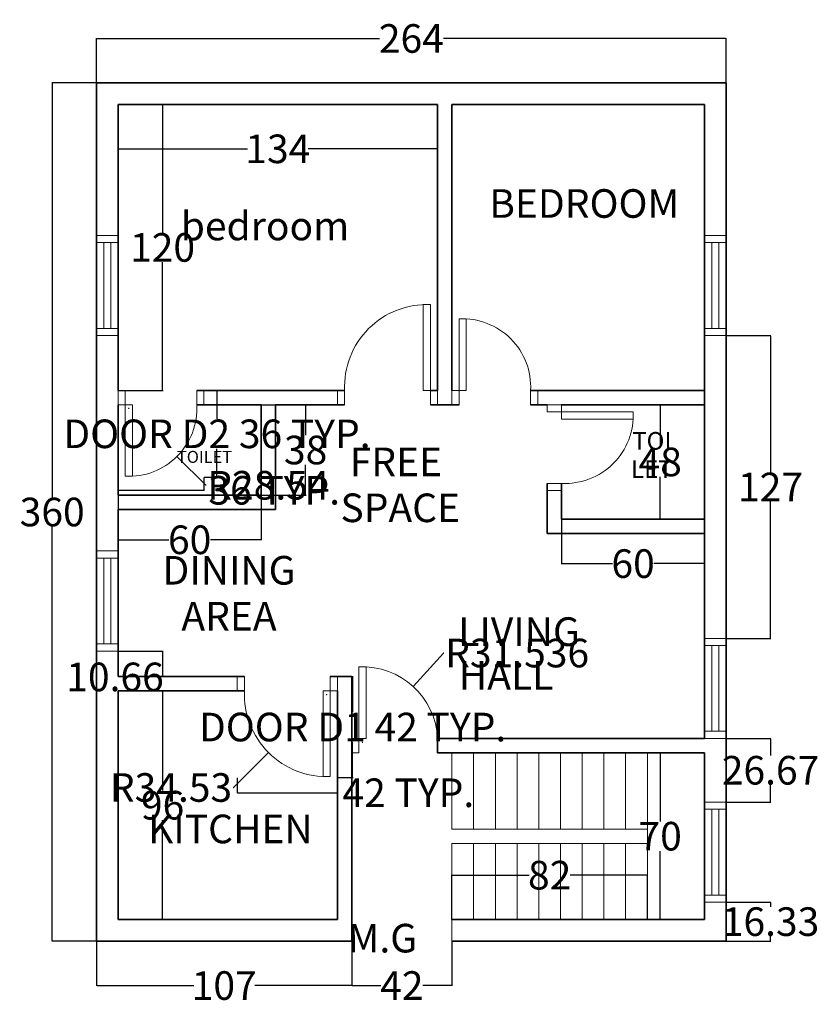
# Model space of a CAD drawing. Units: inches. Extents: x -24 to 1692, y -109 to 592.
# Tile 3 of 4: x 906 to 1241, y 10 to 423. Entities that reach past the tile are written whole.
import ezdxf
from ezdxf.enums import TextEntityAlignment as Align

# ---------------------------------------------------------------- set-up
doc = ezdxf.new("R2010")
doc.units = ezdxf.units.IN
doc.header["$MEASUREMENT"] = 0
for name, color, linetype, lineweight in [('A-ANNO-DIMS', 2, 'Continuous', 18), ('A-ANNO-TEXT', 7, 'Continuous', 18), ('A-AREA-IDEN', 7, 'Continuous', 18), ('A-DOOR', 3, 'Continuous', 18), ('A-FLOR-STRS', 2, 'Continuous', 18), ('A-GLAZ', 4, 'Continuous', 18), ('A-WALL', 7, 'Continuous', 35)]:
    doc.layers.add(name, color=color, linetype=linetype, lineweight=lineweight)
doc.styles.get("Standard").update_dxf_attribs({"font": 'arial.ttf'})
doc.dimstyles.get("Standard").update_dxf_attribs({"dimtxt": 12, "dimasz": 0.18, "dimexe": 0.18, "dimexo": 0.0625, "dimgap": 0.09, "dimtad": 0, "dimtih": 1, "dimtoh": 1, "dimdec": 0, "dimzin": 0, "dimdsep": 46, "dimlunit": 4, "dimtxsty": 'Standard', "dimcen": 0.09, "dimadec": 0, "dimazin": 0, "dimtfac": 1, "dimtdec": 0, "dimtofl": 0, "dimtmove": 0, "dimatfit": 3, "dimfxl": 1, "dimtolj": 1, "dimtzin": 0, "dimarcsym": 0})

# ---------------------------------------------------------------- blocks, each defined once
blk = doc.blocks.new('K')
for p, q in [((0, 42), (9, 42)), ((0, 3), (0, 39)), ((0, 39), (9, 39)), ((3, 3), (3, 39)), ((6, 39), (6, 3)), ((9, 39), (9, 3)), ((9, 3), (0, 3)), ((9, 0), (0, 0))]:
    blk.add_line(p, q)
blk = doc.blocks.new('DOOR-SWING-36IN')
for p, q in [((-39, 0), (-39, 6)), ((-36, 0), (-36, 6)), ((0, 0), (0, 6)), ((3, 0), (3, 6))]:
    blk.add_line(p, q)
blk.add_lwpolyline([(0, 0), (-3, 0), (-3, -36), (0, -36)], close=True)
blk.add_arc((-1.5, -1.5), 34.53, 177.5104, 272.4896)
blk = doc.blocks.new('DOOR-SWING-30IN')
for p, q in [((-3, 6), (-3, 0)), ((0, 6), (0, 0)), ((30, 6), (30, 0)), ((33, 6), (33, 0))]:
    blk.add_line(p, q)
blk.add_lwpolyline([(0, 0), (3, 0), (3, -30), (0, -30)], close=True)
blk.add_arc((1.5, -1.5), 28.54, 266.9872, 3.0128)
blk = doc.blocks.new('*D7')
at = {"layer": 'A-ANNO-DIMS', "color": 0, "lineweight": -2, "transparency": 16777216}
for p, q in [((1039.42, 147.42), (1045.9, 147.42)), ((1045.72, 147.24), (1045.72, 132.51)), ((1045.72, 105.18), (1045.72, 119.91)), ((1039.42, 105), (1045.9, 105))]:
    blk.add_line(p, q, dxfattribs=at)
at = {"layer": 'A-ANNO-DIMS', "color": 0, "transparency": 16777216}
for points in [[(1045.69, 147.24), (1045.75, 147.24), (1045.72, 147.42)], [(1045.69, 105.18), (1045.75, 105.18), (1045.72, 105)]]:
    blk.add_solid(points, dxfattribs=at)
at = {"layer": 'Defpoints', "color": 0, "transparency": 16777216}
for p in [(1039.36, 147.42), (1045.72, 147.42), (1039.36, 105)]:
    blk.add_point(p, dxfattribs=at)
at = {"layer": 'A-ANNO-DIMS', "color": 0, "transparency": 16777216, "insert": (1045.72, 126.21), "char_height": 12, "attachment_point": 5}
blk.add_mtext('\\A1;DOOR D1 42 TYP.', dxfattribs=at)
blk = doc.blocks.new('*D8')
at = {"layer": 'A-ANNO-DIMS', "color": 0, "lineweight": -2, "transparency": 16777216}
for p, q in [((997.36, 104.94), (997.36, 98.46)), ((1039.36, 104.94), (1039.36, 98.46)), ((997.54, 98.64), (1039.18, 98.64)), ((1039.36, 98.64), (1039.54, 98.64))]:
    blk.add_line(p, q, dxfattribs=at)
at = {"layer": 'A-ANNO-DIMS', "color": 0, "transparency": 16777216}
for points in [[(997.54, 98.67), (997.54, 98.61), (997.36, 98.64)], [(1039.18, 98.67), (1039.18, 98.61), (1039.36, 98.64)]]:
    blk.add_solid(points, dxfattribs=at)
at = {"layer": 'Defpoints', "color": 0, "transparency": 16777216}
for p in [(997.36, 105), (1039.36, 105), (1039.36, 98.64)]:
    blk.add_point(p, dxfattribs=at)
at = {"layer": 'A-ANNO-DIMS', "color": 0, "transparency": 16777216, "insert": (1069.08, 98.64), "char_height": 12, "attachment_point": 5}
blk.add_mtext('\\A1;42 TYP.', dxfattribs=at)
blk = doc.blocks.new('*D9')
at = {"layer": 'A-ANNO-DIMS', "color": 0, "lineweight": -2, "transparency": 16777216}
for p, q in [((983.42, 267.42), (989, 267.42)), ((988.82, 267.24), (988.82, 255.51)), ((988.82, 231.17), (988.82, 242.9)), ((983.42, 230.99), (989, 230.99))]:
    blk.add_line(p, q, dxfattribs=at)
at = {"layer": 'A-ANNO-DIMS', "color": 0, "transparency": 16777216}
for points in [[(988.79, 267.24), (988.85, 267.24), (988.82, 267.42)], [(988.79, 231.17), (988.85, 231.17), (988.82, 230.99)]]:
    blk.add_solid(points, dxfattribs=at)
at = {"layer": 'Defpoints', "color": 0, "transparency": 16777216}
for p in [(983.36, 267.42), (988.82, 267.42), (983.36, 230.99)]:
    blk.add_point(p, dxfattribs=at)
at = {"layer": 'A-ANNO-DIMS', "color": 0, "transparency": 16777216, "insert": (988.82, 249.21), "char_height": 12, "attachment_point": 5}
blk.add_mtext('\\A1;DOOR D2 36 TYP.', dxfattribs=at)
blk = doc.blocks.new('*D10')
at = {"layer": 'A-ANNO-DIMS', "color": 0, "lineweight": -2, "transparency": 16777216}
for p, q in [((947.36, 230.93), (947.36, 225.35)), ((983.36, 230.93), (983.36, 225.35)), ((947.54, 225.53), (983.18, 225.53)), ((983.36, 225.53), (983.54, 225.53))]:
    blk.add_line(p, q, dxfattribs=at)
at = {"layer": 'A-ANNO-DIMS', "color": 0, "transparency": 16777216}
for points in [[(947.54, 225.56), (947.54, 225.5), (947.36, 225.53)], [(983.18, 225.56), (983.18, 225.5), (983.36, 225.53)]]:
    blk.add_solid(points, dxfattribs=at)
at = {"layer": 'Defpoints', "color": 0, "transparency": 16777216}
for p in [(947.36, 230.99), (983.36, 230.99), (983.36, 225.53)]:
    blk.add_point(p, dxfattribs=at)
at = {"layer": 'A-ANNO-DIMS', "color": 0, "transparency": 16777216, "insert": (1012.83, 225.53), "char_height": 12, "attachment_point": 5}
blk.add_mtext('\\A1;36 TYP.', dxfattribs=at)
blk = doc.blocks.new('*D55')
at = {"layer": 'A-ANNO-DIMS', "color": 0, "lineweight": -2, "transparency": 16777216}
for p, q in [((938.36, 396.48), (938.36, 415.25)), ((938.54, 415.07), (1056.93, 415.07)), ((1202.18, 415.07), (1083.78, 415.07)), ((1202.36, 396.48), (1202.36, 415.25))]:
    blk.add_line(p, q, dxfattribs=at)
at = {"layer": 'A-ANNO-DIMS', "color": 0, "transparency": 16777216}
for points in [[(938.54, 415.1), (938.54, 415.04), (938.36, 415.07)], [(1202.18, 415.1), (1202.18, 415.04), (1202.36, 415.07)]]:
    blk.add_solid(points, dxfattribs=at)
at = {"layer": 'Defpoints', "color": 0, "transparency": 16777216}
for p in [(1202.36, 415.07), (938.36, 396.42), (1202.36, 396.42)]:
    blk.add_point(p, dxfattribs=at)
at = {"layer": 'A-ANNO-DIMS', "color": 0, "transparency": 16777216, "insert": (1070.36, 415.07), "char_height": 12, "attachment_point": 5}
blk.add_mtext('\\A1;264', dxfattribs=at)
blk = doc.blocks.new('*D56')
at = {"layer": 'A-ANNO-DIMS', "color": 0, "lineweight": -2, "transparency": 16777216}
for p, q in [((938.3, 396.42), (919.53, 396.42)), ((919.71, 396.24), (919.71, 222.64)), ((919.71, 36.6), (919.71, 210.2)), ((938.3, 36.42), (919.53, 36.42))]:
    blk.add_line(p, q, dxfattribs=at)
at = {"layer": 'A-ANNO-DIMS', "color": 0, "transparency": 16777216}
for points in [[(919.68, 396.24), (919.74, 396.24), (919.71, 396.42)], [(919.68, 36.6), (919.74, 36.6), (919.71, 36.42)]]:
    blk.add_solid(points, dxfattribs=at)
at = {"layer": 'Defpoints', "color": 0, "transparency": 16777216}
for p in [(919.71, 396.42), (938.36, 396.42), (938.36, 36.42)]:
    blk.add_point(p, dxfattribs=at)
at = {"layer": 'A-ANNO-DIMS', "color": 0, "transparency": 16777216, "insert": (919.71, 216.42), "char_height": 12, "attachment_point": 5}
blk.add_mtext('\\A1;360', dxfattribs=at)
blk = doc.blocks.new('*D57')
at = {"layer": 'A-ANNO-DIMS', "color": 0, "lineweight": -2, "transparency": 16777216}
for p, q in [((947.36, 387.36), (947.36, 368.59)), ((1081.36, 387.36), (1081.36, 368.59)), ((947.54, 368.77), (1001.6, 368.77)), ((1081.18, 368.77), (1027.12, 368.77))]:
    blk.add_line(p, q, dxfattribs=at)
at = {"layer": 'A-ANNO-DIMS', "color": 0, "transparency": 16777216}
for points in [[(947.54, 368.8), (947.54, 368.74), (947.36, 368.77)], [(1081.18, 368.8), (1081.18, 368.74), (1081.36, 368.77)]]:
    blk.add_solid(points, dxfattribs=at)
at = {"layer": 'Defpoints', "color": 0, "transparency": 16777216}
for p in [(947.36, 387.42), (1081.36, 387.42), (947.36, 368.77)]:
    blk.add_point(p, dxfattribs=at)
at = {"layer": 'A-ANNO-DIMS', "color": 0, "transparency": 16777216, "insert": (1014.36, 368.77), "char_height": 12, "attachment_point": 5}
blk.add_mtext('\\A1;134', dxfattribs=at)
blk = doc.blocks.new('*D58')
at = {"layer": 'A-ANNO-DIMS', "color": 0, "lineweight": -2, "transparency": 16777216}
for p, q in [((947.42, 387.42), (966.19, 387.42)), ((966.01, 387.24), (966.01, 333.64)), ((966.01, 267.6), (966.01, 321.2)), ((947.42, 267.42), (966.19, 267.42))]:
    blk.add_line(p, q, dxfattribs=at)
at = {"layer": 'A-ANNO-DIMS', "color": 0, "transparency": 16777216}
for points in [[(965.98, 387.24), (966.04, 387.24), (966.01, 387.42)], [(965.98, 267.6), (966.04, 267.6), (966.01, 267.42)]]:
    blk.add_solid(points, dxfattribs=at)
at = {"layer": 'Defpoints', "color": 0, "transparency": 16777216}
for p in [(947.36, 387.42), (947.36, 267.42), (966.01, 267.42)]:
    blk.add_point(p, dxfattribs=at)
at = {"layer": 'A-ANNO-DIMS', "color": 0, "transparency": 16777216, "insert": (966.01, 327.42), "char_height": 12, "attachment_point": 5}
blk.add_mtext('\\A1;120', dxfattribs=at)
blk = doc.blocks.new('*D59')
at = {"layer": 'A-ANNO-DIMS', "color": 0, "lineweight": -2, "transparency": 16777216}
for p, q in [((938.36, 36.36), (938.36, 17.59)), ((1045.36, 36.36), (1045.36, 17.59)), ((938.54, 17.77), (979.08, 17.77)), ((1045.18, 17.77), (1004.64, 17.77))]:
    blk.add_line(p, q, dxfattribs=at)
at = {"layer": 'A-ANNO-DIMS', "color": 0, "transparency": 16777216}
for points in [[(938.54, 17.8), (938.54, 17.74), (938.36, 17.77)], [(1045.18, 17.8), (1045.18, 17.74), (1045.36, 17.77)]]:
    blk.add_solid(points, dxfattribs=at)
at = {"layer": 'Defpoints', "color": 0, "transparency": 16777216}
for p in [(938.36, 36.42), (1045.36, 36.42), (1045.36, 17.77)]:
    blk.add_point(p, dxfattribs=at)
at = {"layer": 'A-ANNO-DIMS', "color": 0, "transparency": 16777216, "insert": (991.86, 17.77), "char_height": 12, "attachment_point": 5}
blk.add_mtext('\\A1;107', dxfattribs=at)
blk = doc.blocks.new('*D60')
at = {"layer": 'A-ANNO-DIMS', "color": 0, "lineweight": -2, "transparency": 16777216}
for p, q in [((1045.36, 36.36), (1045.36, 17.59)), ((1087.36, 36.36), (1087.36, 17.59)), ((1045.54, 17.77), (1057.49, 17.77)), ((1087.18, 17.77), (1075.22, 17.77))]:
    blk.add_line(p, q, dxfattribs=at)
at = {"layer": 'A-ANNO-DIMS', "color": 0, "transparency": 16777216}
for points in [[(1045.54, 17.8), (1045.54, 17.74), (1045.36, 17.77)], [(1087.18, 17.8), (1087.18, 17.74), (1087.36, 17.77)]]:
    blk.add_solid(points, dxfattribs=at)
at = {"layer": 'Defpoints', "color": 0, "transparency": 16777216}
for p in [(1045.36, 36.42), (1087.36, 36.42), (1087.36, 17.77)]:
    blk.add_point(p, dxfattribs=at)
at = {"layer": 'A-ANNO-DIMS', "color": 0, "transparency": 16777216, "insert": (1066.36, 17.77), "char_height": 12, "attachment_point": 5}
blk.add_mtext('\\A1;42', dxfattribs=at)
blk = doc.blocks.new('*D61')
at = {"layer": 'A-ANNO-DIMS', "color": 0, "lineweight": -2, "transparency": 16777216}
for p, q in [((947.42, 141.42), (966.19, 141.42)), ((966.01, 141.24), (966.01, 99.64)), ((966.01, 45.6), (966.01, 87.2)), ((947.42, 45.42), (966.19, 45.42))]:
    blk.add_line(p, q, dxfattribs=at)
at = {"layer": 'A-ANNO-DIMS', "color": 0, "transparency": 16777216}
for points in [[(965.98, 141.24), (966.04, 141.24), (966.01, 141.42)], [(965.98, 45.6), (966.04, 45.6), (966.01, 45.42)]]:
    blk.add_solid(points, dxfattribs=at)
at = {"layer": 'Defpoints', "color": 0, "transparency": 16777216}
for p in [(947.36, 141.42), (947.36, 45.42), (966.01, 45.42)]:
    blk.add_point(p, dxfattribs=at)
at = {"layer": 'A-ANNO-DIMS', "color": 0, "transparency": 16777216, "insert": (966.01, 93.42), "char_height": 12, "attachment_point": 5}
blk.add_mtext('\\A1;96', dxfattribs=at)
blk = doc.blocks.new('*D62')
at = {"layer": 'A-ANNO-DIMS', "color": 0, "lineweight": -2, "transparency": 16777216}
for p, q in [((1193.3, 115.42), (1174.53, 115.42)), ((1174.71, 115.24), (1174.71, 86.64)), ((1174.71, 45.6), (1174.71, 74.2)), ((1193.3, 45.42), (1174.53, 45.42))]:
    blk.add_line(p, q, dxfattribs=at)
at = {"layer": 'A-ANNO-DIMS', "color": 0, "transparency": 16777216}
for points in [[(1174.68, 115.24), (1174.74, 115.24), (1174.71, 115.42)], [(1174.68, 45.6), (1174.74, 45.6), (1174.71, 45.42)]]:
    blk.add_solid(points, dxfattribs=at)
at = {"layer": 'Defpoints', "color": 0, "transparency": 16777216}
for p in [(1174.71, 115.42), (1193.36, 115.42), (1193.36, 45.42)]:
    blk.add_point(p, dxfattribs=at)
at = {"layer": 'A-ANNO-DIMS', "color": 0, "transparency": 16777216, "insert": (1174.71, 80.42), "char_height": 12, "attachment_point": 5}
blk.add_mtext('\\A1;70', dxfattribs=at)
blk = doc.blocks.new('*D63')
at = {"layer": 'A-ANNO-DIMS', "color": 0, "lineweight": -2, "transparency": 16777216}
for p, q in [((947.36, 223.36), (947.36, 204.59)), ((1007.36, 223.36), (1007.36, 204.59)), ((947.54, 204.77), (968.66, 204.77)), ((1007.18, 204.77), (986.06, 204.77))]:
    blk.add_line(p, q, dxfattribs=at)
at = {"layer": 'A-ANNO-DIMS', "color": 0, "transparency": 16777216}
for points in [[(947.54, 204.8), (947.54, 204.74), (947.36, 204.77)], [(1007.18, 204.8), (1007.18, 204.74), (1007.36, 204.77)]]:
    blk.add_solid(points, dxfattribs=at)
at = {"layer": 'Defpoints', "color": 0, "transparency": 16777216}
for p in [(947.36, 223.42), (1007.36, 223.42), (947.36, 204.77)]:
    blk.add_point(p, dxfattribs=at)
at = {"layer": 'A-ANNO-DIMS', "color": 0, "transparency": 16777216, "insert": (977.36, 204.77), "char_height": 12, "attachment_point": 5}
blk.add_mtext('\\A1;60', dxfattribs=at)
blk = doc.blocks.new('*D64')
at = {"layer": 'A-ANNO-DIMS', "color": 0, "lineweight": -2, "transparency": 16777216}
for p, q in [((1007.42, 261.42), (1026.19, 261.42)), ((1026.01, 261.24), (1026.01, 248.64)), ((1026.01, 223.6), (1026.01, 236.2)), ((1007.42, 223.42), (1026.19, 223.42))]:
    blk.add_line(p, q, dxfattribs=at)
at = {"layer": 'A-ANNO-DIMS', "color": 0, "transparency": 16777216}
for points in [[(1025.98, 261.24), (1026.04, 261.24), (1026.01, 261.42)], [(1025.98, 223.6), (1026.04, 223.6), (1026.01, 223.42)]]:
    blk.add_solid(points, dxfattribs=at)
at = {"layer": 'Defpoints', "color": 0, "transparency": 16777216}
for p in [(1007.36, 261.42), (1007.36, 223.42), (1026.01, 223.42)]:
    blk.add_point(p, dxfattribs=at)
at = {"layer": 'A-ANNO-DIMS', "color": 0, "transparency": 16777216, "insert": (1026.01, 242.42), "char_height": 12, "attachment_point": 5}
blk.add_mtext('\\A1;38', dxfattribs=at)
blk = doc.blocks.new('*D65')
at = {"layer": 'A-ANNO-DIMS', "color": 0, "lineweight": -2, "transparency": 16777216}
for p, q in [((1133.36, 213.36), (1133.36, 194.59)), ((1193.36, 213.36), (1193.36, 194.59)), ((1133.54, 194.77), (1154.66, 194.77)), ((1193.18, 194.77), (1172.06, 194.77))]:
    blk.add_line(p, q, dxfattribs=at)
at = {"layer": 'A-ANNO-DIMS', "color": 0, "transparency": 16777216}
for points in [[(1133.54, 194.8), (1133.54, 194.74), (1133.36, 194.77)], [(1193.18, 194.8), (1193.18, 194.74), (1193.36, 194.77)]]:
    blk.add_solid(points, dxfattribs=at)
at = {"layer": 'Defpoints', "color": 0, "transparency": 16777216}
for p in [(1133.36, 213.42), (1193.36, 213.42), (1133.36, 194.77)]:
    blk.add_point(p, dxfattribs=at)
at = {"layer": 'A-ANNO-DIMS', "color": 0, "transparency": 16777216, "insert": (1163.36, 194.77), "char_height": 12, "attachment_point": 5}
blk.add_mtext('\\A1;60', dxfattribs=at)
blk = doc.blocks.new('*D66')
at = {"layer": 'A-ANNO-DIMS', "color": 0, "lineweight": -2, "transparency": 16777216}
for p, q in [((1193.3, 261.42), (1174.53, 261.42)), ((1174.71, 261.24), (1174.71, 243.64)), ((1174.71, 213.6), (1174.71, 231.2)), ((1193.3, 213.42), (1174.53, 213.42))]:
    blk.add_line(p, q, dxfattribs=at)
at = {"layer": 'A-ANNO-DIMS', "color": 0, "transparency": 16777216}
for points in [[(1174.68, 261.24), (1174.74, 261.24), (1174.71, 261.42)], [(1174.68, 213.6), (1174.74, 213.6), (1174.71, 213.42)]]:
    blk.add_solid(points, dxfattribs=at)
at = {"layer": 'Defpoints', "color": 0, "transparency": 16777216}
for p in [(1174.71, 261.42), (1193.36, 261.42), (1193.36, 213.42)]:
    blk.add_point(p, dxfattribs=at)
at = {"layer": 'A-ANNO-DIMS', "color": 0, "transparency": 16777216, "insert": (1174.71, 237.42), "char_height": 12, "attachment_point": 5}
blk.add_mtext('\\A1;48', dxfattribs=at)
blk = doc.blocks.new('*D67')
at = {"layer": 'A-ANNO-DIMS', "color": 0, "lineweight": -2, "transparency": 16777216}
for p, q in [((1202.42, 290.41), (1221.19, 290.41)), ((1221.01, 290.23), (1221.01, 233.03)), ((1221.01, 163.6), (1221.01, 220.8)), ((1202.42, 163.42), (1221.19, 163.42))]:
    blk.add_line(p, q, dxfattribs=at)
at = {"layer": 'A-ANNO-DIMS', "color": 0, "transparency": 16777216}
for points in [[(1220.98, 290.23), (1221.04, 290.23), (1221.01, 290.41)], [(1220.98, 163.6), (1221.04, 163.6), (1221.01, 163.42)]]:
    blk.add_solid(points, dxfattribs=at)
at = {"layer": 'Defpoints', "color": 0, "transparency": 16777216}
for p in [(1202.36, 290.41), (1221.01, 290.41), (1202.36, 163.42)]:
    blk.add_point(p, dxfattribs=at)
at = {"layer": 'A-ANNO-DIMS', "color": 0, "transparency": 16777216, "insert": (1221.01, 226.92), "char_height": 12, "attachment_point": 5}
blk.add_mtext('\\A1;127', dxfattribs=at)
blk = doc.blocks.new('*D68')
at = {"layer": 'A-ANNO-DIMS', "color": 0, "lineweight": -2, "transparency": 16777216}
for p, q in [((947.42, 158.08), (966.19, 158.08)), ((966.01, 157.9), (966.01, 147.6)), ((947.42, 147.42), (966.19, 147.42)), ((966.01, 147.24), (965.83, 147.24)), ((966.01, 147.42), (966.01, 147.24))]:
    blk.add_line(p, q, dxfattribs=at)
at = {"layer": 'A-ANNO-DIMS', "color": 0, "transparency": 16777216}
for points in [[(965.98, 157.9), (966.04, 157.9), (966.01, 158.08)], [(965.98, 147.6), (966.04, 147.6), (966.01, 147.42)]]:
    blk.add_solid(points, dxfattribs=at)
at = {"layer": 'Defpoints', "color": 0, "transparency": 16777216}
for p in [(947.36, 158.08), (947.36, 147.42), (966.01, 147.42)]:
    blk.add_point(p, dxfattribs=at)
at = {"layer": 'A-ANNO-DIMS', "color": 0, "transparency": 16777216, "insert": (946.06, 147.24), "char_height": 12, "attachment_point": 5}
blk.add_mtext('\\A1;10.66', dxfattribs=at)
blk = doc.blocks.new('*D69')
at = {"layer": 'A-ANNO-DIMS', "color": 0, "lineweight": -2, "transparency": 16777216}
for p, q in [((1202.42, 52.75), (1221.19, 52.75)), ((1221.01, 52.57), (1221.01, 50.81)), ((1221.01, 36.6), (1221.01, 38.36)), ((1202.42, 36.42), (1221.19, 36.42))]:
    blk.add_line(p, q, dxfattribs=at)
at = {"layer": 'A-ANNO-DIMS', "color": 0, "transparency": 16777216}
for points in [[(1220.98, 52.57), (1221.04, 52.57), (1221.01, 52.75)], [(1220.98, 36.6), (1221.04, 36.6), (1221.01, 36.42)]]:
    blk.add_solid(points, dxfattribs=at)
at = {"layer": 'Defpoints', "color": 0, "transparency": 16777216}
for p in [(1202.36, 52.75), (1221.01, 52.75), (1202.36, 36.42)]:
    blk.add_point(p, dxfattribs=at)
at = {"layer": 'A-ANNO-DIMS', "color": 0, "transparency": 16777216, "insert": (1221.01, 44.58), "char_height": 12, "attachment_point": 5}
blk.add_mtext('\\A1;16.33', dxfattribs=at)
blk = doc.blocks.new('*D70')
at = {"layer": 'A-ANNO-DIMS', "color": 0, "lineweight": -2, "transparency": 16777216}
for p, q in [((1202.42, 121.42), (1221.19, 121.42)), ((1221.01, 121.24), (1221.01, 114.3)), ((1221.01, 94.93), (1221.01, 101.87)), ((1202.42, 94.75), (1221.19, 94.75))]:
    blk.add_line(p, q, dxfattribs=at)
at = {"layer": 'A-ANNO-DIMS', "color": 0, "transparency": 16777216}
for points in [[(1220.98, 121.24), (1221.04, 121.24), (1221.01, 121.42)], [(1220.98, 94.93), (1221.04, 94.93), (1221.01, 94.75)]]:
    blk.add_solid(points, dxfattribs=at)
at = {"layer": 'Defpoints', "color": 0, "transparency": 16777216}
for p in [(1202.36, 121.42), (1221.01, 121.42), (1202.36, 94.75)]:
    blk.add_point(p, dxfattribs=at)
at = {"layer": 'A-ANNO-DIMS', "color": 0, "transparency": 16777216, "insert": (1221.01, 108.08), "char_height": 12, "attachment_point": 5}
blk.add_mtext('\\A1;26.67', dxfattribs=at)
blk = doc.blocks.new('*D71')
at = {"layer": 'A-ANNO-DIMS', "color": 0, "lineweight": -2, "transparency": 16777216}
for p, q in [((1087.36, 45.48), (1087.36, 64.25)), ((1087.54, 64.07), (1119.73, 64.07)), ((1169.18, 64.07), (1136.99, 64.07)), ((1169.36, 45.48), (1169.36, 64.25))]:
    blk.add_line(p, q, dxfattribs=at)
at = {"layer": 'A-ANNO-DIMS', "color": 0, "transparency": 16777216}
for points in [[(1087.54, 64.1), (1087.54, 64.04), (1087.36, 64.07)], [(1169.18, 64.1), (1169.18, 64.04), (1169.36, 64.07)]]:
    blk.add_solid(points, dxfattribs=at)
at = {"layer": 'Defpoints', "color": 0, "transparency": 16777216}
for p in [(1169.36, 64.07), (1087.36, 45.42), (1169.36, 45.42)]:
    blk.add_point(p, dxfattribs=at)
at = {"layer": 'A-ANNO-DIMS', "color": 0, "transparency": 16777216, "insert": (1128.36, 64.07), "char_height": 12, "attachment_point": 5}
blk.add_mtext('\\A1;82', dxfattribs=at)
blk = doc.blocks.new('*D97')
at = {"layer": 'A-ANNO-DIMS', "color": 0, "lineweight": -2, "transparency": 16777216}
for p, q in [((1034.77, 139.92), (1034.95, 139.92)), ((1034.86, 139.83), (1034.86, 140.01)), ((995.79, 100.85), (1010.31, 115.37)), ((995.61, 100.85), (995.79, 100.85))]:
    blk.add_line(p, q, dxfattribs=at)
at = {"layer": 'A-ANNO-DIMS', "color": 0, "transparency": 16777216}
blk.add_solid([(1010.29, 115.4), (1010.33, 115.35), (1010.44, 115.5)], dxfattribs=at)
at = {"layer": 'Defpoints', "color": 0, "transparency": 16777216}
for p in [(1034.86, 139.92), (1010.44, 115.5)]:
    blk.add_point(p, dxfattribs=at)
at = {"layer": 'A-ANNO-DIMS', "color": 0, "transparency": 16777216, "insert": (969.53, 100.85), "char_height": 12, "attachment_point": 5}
blk.add_mtext('\\A1;R34.53', dxfattribs=at)
blk = doc.blocks.new('*D98')
at = {"layer": 'A-ANNO-DIMS', "color": 0, "lineweight": -2, "transparency": 16777216}
for p, q in [((1083.8, 157.25), (1071.19, 143.39)), ((1083.98, 157.25), (1083.8, 157.25)), ((1049.77, 119.92), (1049.95, 119.92)), ((1049.86, 119.83), (1049.86, 120.01))]:
    blk.add_line(p, q, dxfattribs=at)
at = {"layer": 'A-ANNO-DIMS', "color": 0, "transparency": 16777216}
blk.add_solid([(1071.17, 143.41), (1071.22, 143.37), (1071.07, 143.25)], dxfattribs=at)
at = {"layer": 'Defpoints', "color": 0, "transparency": 16777216}
for p in [(1071.07, 143.25), (1049.86, 119.92)]:
    blk.add_point(p, dxfattribs=at)
at = {"layer": 'A-ANNO-DIMS', "color": 0, "transparency": 16777216, "insert": (1114.72, 157.25), "char_height": 12, "attachment_point": 5}
blk.add_mtext('\\A1;R31.536', dxfattribs=at)
blk = doc.blocks.new('*D99')
at = {"layer": 'A-ANNO-DIMS', "color": 0, "lineweight": -2, "transparency": 16777216}
for p, q in [((951.77, 259.92), (951.95, 259.92)), ((951.86, 259.83), (951.86, 260.01)), ((984.15, 227.63), (972.17, 239.61)), ((984.33, 227.63), (984.15, 227.63))]:
    blk.add_line(p, q, dxfattribs=at)
at = {"layer": 'A-ANNO-DIMS', "color": 0, "transparency": 16777216}
blk.add_solid([(972.19, 239.63), (972.14, 239.59), (972.04, 239.74)], dxfattribs=at)
at = {"layer": 'Defpoints', "color": 0, "transparency": 16777216}
for p in [(951.86, 259.92), (972.04, 239.74)]:
    blk.add_point(p, dxfattribs=at)
at = {"layer": 'A-ANNO-DIMS', "color": 0, "transparency": 16777216, "insert": (1010.38, 227.63), "char_height": 12, "attachment_point": 5}
blk.add_mtext('\\A1;R28.54', dxfattribs=at)

msp = doc.modelspace()

# ---------------------------------------------------------------- linework, layer by layer
at = {"layer": 'A-DOOR'}
for p, q in [((950.3585, 267.4197), (947.3585, 267.4197)), ((950.3585, 267.4197), (947.3585, 267.4197)), ((1090.3585, 267.4197), (1087.3585, 267.4197)), ((950.3585, 261.4197), (947.3585, 261.4197)), ((1127.3585, 258.4197), (1127.3585, 261.4197)), ((1133.3585, 255.4197), (1133.3585, 261.4197)), ((1036.3585, 141.4197), (1039.3585, 141.4197)), ((1045.3585, 121.4197), (1045.3585, 115.4197)), ((1048.3585, 121.4197), (1045.3585, 121.4197)), ((1048.3585, 121.4197), (1048.3585, 115.4197)), ((1048.3585, 115.4197), (1045.3585, 115.4197))]:
    msp.add_line(p, q, dxfattribs=at)
msp.add_lwpolyline([(1048.3585, 121.4197), (1051.3585, 121.4197), (1051.3585, 151.4197), (1048.3585, 151.4197)], close=True, dxfattribs=at)
msp.add_arc((1049.8585, 119.9197), 31.5357, 2.726311, 92.726311, dxfattribs=at)
at = {"layer": 'A-FLOR-STRS'}
for p, q in [((1087.3585, 115.4197), (1087.3585, 83.4197)), ((1096.4685, 115.4197), (1096.4685, 83.4197)), ((1105.5785, 115.4197), (1105.5785, 83.4197)), ((1114.6885, 115.4197), (1114.6885, 83.4197)), ((1123.7985, 115.4197), (1123.7985, 83.4197)), ((1132.9085, 115.4197), (1132.9085, 83.4197)), ((1142.0185, 115.4197), (1142.0185, 83.4197)), ((1151.1285, 115.4197), (1151.1285, 83.4197)), ((1160.2385, 115.4197), (1160.2385, 83.4197)), ((1169.3585, 45.4197), (1169.3585, 115.4197)), ((1169.3585, 83.4197), (1087.3585, 83.4197)), ((1087.3585, 77.4197), (1169.3585, 77.4197)), ((1087.3585, 77.4197), (1087.3585, 36.4197)), ((1096.4685, 77.4197), (1096.4685, 45.4197)), ((1105.5785, 77.4197), (1105.5785, 45.4197)), ((1114.6885, 77.4197), (1114.6885, 45.4197)), ((1123.7985, 77.4197), (1123.7985, 45.4197)), ((1132.9085, 77.4197), (1132.9085, 45.4197)), ((1142.0185, 77.4197), (1142.0185, 45.4197)), ((1151.1285, 77.4197), (1151.1285, 45.4197)), ((1160.2385, 77.4197), (1160.2385, 45.4197))]:
    msp.add_line(p, q, dxfattribs=at)
msp.add_lwpolyline([(1100.5256, 97.8368, 0, 0, 0), (1178.3724, 97.8368, 0, 0, 0), (1178.3724, 57.6767, 0, 0, 0), (1137.4138, 57.6767, 12, 0, 0), (1110.4472, 57.6767, 0, 0, 0)], format="xyseb", dxfattribs=at)
at = {"layer": 'A-WALL'}
for p, q in [((947.3585, 387.4197), (947.3585, 267.4197)), ((1007.3585, 387.4197), (947.3585, 387.4197)), ((1081.3585, 387.4197), (947.3585, 387.4197)), ((1081.3585, 387.4197), (1081.3585, 267.4197)), ((1193.3585, 387.4197), (1087.3585, 387.4197)), ((1087.3585, 387.4197), (1087.3585, 267.4197)), ((1127.3585, 387.4197), (1087.3585, 387.4197)), ((1193.3585, 121.4197), (1193.3585, 387.4197)), ((1007.3585, 267.4197), (980.3585, 267.4197)), ((1042.3585, 267.4197), (980.3585, 267.4197)), ((1081.3585, 267.4197), (1078.3585, 267.4197)), ((1193.3585, 267.4197), (1120.3585, 267.4197)), ((1193.3585, 267.4197), (1133.3585, 267.4197)), ((947.3585, 261.4197), (947.3585, 223.4197)), ((1007.3585, 261.4197), (980.3585, 261.4197)), ((1007.3585, 261.4197), (1007.3585, 223.4197)), ((1013.3585, 261.4197), (1013.3585, 217.4197)), ((1042.3585, 261.4197), (1013.3585, 261.4197)), ((1090.3585, 261.4197), (1078.3585, 261.4197)), ((1127.3585, 261.4197), (1120.3585, 261.4197)), ((1193.3585, 261.4197), (1133.3585, 261.4197)), ((1127.3585, 207.4197), (1127.3585, 228.4197)), ((1133.3585, 213.4197), (1133.3585, 228.4197)), ((1007.3585, 223.4197), (947.3585, 223.4197)), ((1013.3585, 217.4197), (947.3585, 217.4197)), ((947.3585, 217.4197), (947.3585, 147.4197)), ((1193.3585, 213.4197), (1133.3585, 213.4197)), ((1193.3585, 207.4197), (1127.3585, 207.4197)), ((947.3585, 147.4197), (1000.3585, 147.4197)), ((1036.3585, 147.4197), (1045.3585, 147.4197)), ((1045.3585, 147.4197), (1045.3585, 36.4197)), ((947.3585, 141.4197), (947.3585, 45.4197)), ((947.3585, 141.4197), (1000.3585, 141.4197)), ((947.3585, 141.4197), (947.3585, 121.4197)), ((1039.3585, 141.4197), (1039.3585, 45.4197)), ((1193.3585, 121.4197), (1081.3585, 121.4197)), ((1081.3585, 121.4197), (1081.3585, 115.4197)), ((1193.3585, 115.4197), (1081.3585, 115.4197)), ((1193.3585, 45.4197), (1193.3585, 115.4197)), ((947.3585, 45.4197), (1039.3585, 45.4197)), ((1087.3585, 45.4197), (1193.3585, 45.4197))]:
    msp.add_line(p, q, dxfattribs=at)
msp.add_lwpolyline([(1087.3585, 36.4197), (1202.3585, 36.4197), (1202.3585, 396.4197), (938.3585, 396.4197), (938.3585, 36.4197), (1045.3585, 36.4197)], dxfattribs=at)

# ---------------------------------------------------------------- block references
at = {"layer": 'A-DOOR', "extrusion": (0, 0, -1), "zscale": -1}
for name, p, rotation in [('DOOR-SWING-36IN', (-1078.3585, 267.4197), 180), ('DOOR-SWING-30IN', (-1090.3585, 267.4197), 180), ('DOOR-SWING-30IN', (-1133.3585, 258.4197), 269.9999999999998)]:
    msp.add_blockref(name, p, dxfattribs=dict(at, rotation=rotation))
at = {"layer": 'A-DOOR'}
for name, p in [('DOOR-SWING-30IN', (950.3585, 261.4197)), ('DOOR-SWING-36IN', (1036.3585, 141.4197))]:
    msp.add_blockref(name, p, dxfattribs=at)
at = {"layer": 'A-GLAZ'}
for p in [(938.3585, 290.4113), (1193.3585, 290.4113), (938.3585, 158.0801), (1193.3585, 121.4197), (1193.3585, 52.7496)]:
    msp.add_blockref('K', p, dxfattribs=at)

# ---------------------------------------------------------------- texts
at = {"layer": 'A-ANNO-TEXT'}
msp.add_text('M.G', height=12, dxfattribs=at).set_placement((1058.2115, 31.6448), align=Align.CENTER)
at = {"layer": 'A-AREA-IDEN'}
for s, height, p in [('BEDROOM', 12, (1142.8616, 339.834)), ('bedroom', 12, (1008.9859, 330.4144)), ('TOI', 7.38227, (1171.2162, 242.5855)), ('TOILET', 5.03555, (983.5946, 237.0307)), ('FREE ', 12, (1065.7012, 231.4507)), ('LET', 7.38227, (1171.2162, 230.7265)), ('SPACE', 12, (1065.7012, 212.1737)), ('DINING', 12, (993.8666, 185.9717)), ('AREA', 12, (993.8666, 166.6948)), ('LIVING', 12, (1115.4993, 160.2346)), ('HALL', 12, (1110.0852, 141.89)), ('KITCHEN', 12, (994.4303, 77.4606))]:
    msp.add_text(s, height=height, dxfattribs=at).set_placement(p, align=Align.CENTER)

# ---------------------------------------------------------------- dimensions: what is measured, and where the dimension line sits
at = {"layer": 'A-ANNO-DIMS'}
for base, p1, p2, picture, middle in [((1202.3585, 415.0697), (938.3585, 396.4197), (1202.3585, 396.4197), '*D55', (1070.3585, 415.0697)), ((1169.3585, 64.0697), (1087.3585, 45.4197), (1169.3585, 45.4197), '*D71', (1128.3585, 64.0697)), ((1045.3585, 17.7697), (938.3585, 36.4197), (1045.3585, 36.4197), '*D59', (991.8585, 17.7697)), ((1087.3585, 17.7697), (1045.3585, 36.4197), (1087.3585, 36.4197), '*D60', (1066.3585, 17.7697))]:
    dim = msp.add_linear_dim(base=base, p1=p1, p2=p2, dimstyle='Standard', override={"dimdec": 0, "dimlfac": 1, "dimrnd": 0, "dimzin": 0, "dimdsep": 46, "dimlunit": 2}, dxfattribs=at)
    dim.commit()
    dim.dimension.update_dxf_attribs({"geometry": picture, "text_midpoint": middle})
for base, p1, p2, angle, override, picture, middle in [((919.7085, 396.4197), (938.3585, 36.4197), (938.3585, 396.4197), 90, {"dimdec": 0, "dimlfac": 1, "dimrnd": 0, "dimzin": 0, "dimdsep": 46, "dimlunit": 2}, '*D56', (919.7085, 216.4197)), ((947.3585, 368.7697), (1081.3585, 387.4197), (947.3585, 387.4197), 180, {"dimdec": 0, "dimlfac": 1, "dimrnd": 0, "dimzin": 0, "dimdsep": 46, "dimlunit": 2}, '*D57', (1014.3585, 368.7697)), ((966.0085, 267.4197), (947.3585, 387.4197), (947.3585, 267.4197), 270, {"dimdec": 0, "dimlfac": 1, "dimrnd": 0, "dimzin": 0, "dimdsep": 46, "dimlunit": 2}, '*D58', (966.0085, 327.4197)), ((1221.0085, 290.4113), (1202.3585, 163.4197), (1202.3585, 290.4113), 90, {"dimdec": 0, "dimlfac": 1, "dimrnd": 0, "dimzin": 0, "dimdsep": 46, "dimlunit": 2}, '*D67', (1221.0085, 226.9155)), ((1026.0085, 223.4197), (1007.3585, 261.4197), (1007.3585, 223.4197), 270, {"dimdec": 0, "dimlfac": 1, "dimrnd": 0, "dimzin": 0, "dimdsep": 46, "dimlunit": 2}, '*D64', (1026.0085, 242.4197)), ((1174.7085, 261.4197), (1193.3585, 213.4197), (1193.3585, 261.4197), 90, {"dimdec": 0, "dimlfac": 1, "dimrnd": 0, "dimzin": 0, "dimdsep": 46, "dimlunit": 2}, '*D66', (1174.7085, 237.4197)), ((947.3585, 204.7697), (1007.3585, 223.4197), (947.3585, 223.4197), 180, {"dimdec": 0, "dimlfac": 1, "dimrnd": 0, "dimzin": 0, "dimdsep": 46, "dimlunit": 2}, '*D63', (977.3585, 204.7697)), ((1133.3585, 194.7697), (1193.3585, 213.4197), (1133.3585, 213.4197), 180, {"dimdec": 0, "dimlfac": 1, "dimrnd": 0, "dimzin": 0, "dimdsep": 46, "dimlunit": 2}, '*D65', (1163.3585, 194.7697)), ((966.0085, 147.4197), (947.3585, 158.0801), (947.3585, 147.4197), 270, {"dimdec": 2, "dimlfac": 1, "dimrnd": 0, "dimzin": 0, "dimdsep": 46, "dimlunit": 2}, '*D68', (946.0604, 147.2397)), ((966.0085, 45.4197), (947.3585, 141.4197), (947.3585, 45.4197), 270, {"dimdec": 0, "dimlfac": 1, "dimrnd": 0, "dimzin": 0, "dimdsep": 46, "dimlunit": 2}, '*D61', (966.0085, 93.4197)), ((1221.0085, 121.4197), (1202.3585, 94.7496), (1202.3585, 121.4197), 90, {"dimdec": 2, "dimlfac": 1, "dimrnd": 0, "dimzin": 0, "dimdsep": 46, "dimlunit": 2}, '*D70', (1221.0085, 108.0847)), ((1174.7085, 115.4197), (1193.3585, 45.4197), (1193.3585, 115.4197), 90, {"dimdec": 0, "dimlfac": 1, "dimrnd": 0, "dimzin": 0, "dimdsep": 46, "dimlunit": 2}, '*D62', (1174.7085, 80.4197)), ((1221.0085, 52.7496), (1202.3585, 36.4197), (1202.3585, 52.7496), 90, {"dimdec": 2, "dimlfac": 1, "dimrnd": 0, "dimzin": 0, "dimdsep": 46, "dimlunit": 2}, '*D69', (1221.0085, 44.5847))]:
    dim = msp.add_linear_dim(base=base, p1=p1, p2=p2, angle=angle, dimstyle='Standard', override=override, dxfattribs=at)
    dim.commit()
    dim.dimension.update_dxf_attribs({"geometry": picture, "text_midpoint": middle})
for base, p1, p2, text, picture, middle in [((988.8223, 267.4197), (983.3585, 230.9945), (983.3585, 267.4197), 'DOOR D2 <> TYP.', '*D9', (988.8223, 249.2071)), ((1045.7215, 147.4197), (1039.3585, 104.9993), (1039.3585, 147.4197), 'DOOR D1 <> TYP.', '*D7', (1045.7215, 126.2095))]:
    dim = msp.add_linear_dim(base=base, p1=p1, p2=p2, angle=90, text=text, dimstyle='Standard', override={"dimdec": 0, "dimlfac": 1, "dimrnd": 0, "dimzin": 0, "dimdsep": 46, "dimlunit": 2}, dxfattribs=at)
    dim.commit()
    dim.dimension.update_dxf_attribs({"geometry": picture, "text_midpoint": middle})
for center, mpoint, override, picture, middle in [((951.8585, 259.9197), (972.0388, 239.7392), {"dimdec": 2, "dimlfac": 1, "dimrnd": 0, "dimzin": 0, "dimdsep": 46, "dimlunit": 2}, '*D99', (1010.3815, 227.6309)), ((1049.8585, 119.9197), (1071.072, 143.254), {"dimdec": 3, "dimlfac": 1, "dimrnd": 0, "dimzin": 0, "dimdsep": 46, "dimlunit": 2}, '*D98', (1114.7167, 157.2545)), ((1034.8585, 139.9197), (1010.4404, 115.5014), {"dimdec": 2, "dimlfac": 1, "dimrnd": 0, "dimzin": 0, "dimdsep": 46, "dimlunit": 2}, '*D97', (969.5304, 100.8504))]:
    dim = msp.add_radius_dim(center=center, mpoint=mpoint, dimstyle='Standard', override=override, dxfattribs=at)
    dim.commit()
    dim.dimension.update_dxf_attribs({"geometry": picture, "text_midpoint": middle, "dimtype": 164})
for base, p1, p2, picture, middle in [((983.3585, 225.5307), (947.3585, 230.9945), (983.3585, 230.9945), '*D10', (1012.8304, 225.5307)), ((1039.3585, 98.6362), (997.3585, 104.9993), (1039.3585, 104.9993), '*D8', (1069.0759, 98.6362))]:
    dim = msp.add_linear_dim(base=base, p1=p1, p2=p2, text='<> TYP.', dimstyle='Standard', override={"dimdec": 0, "dimlfac": 1, "dimrnd": 0, "dimzin": 0, "dimdsep": 46, "dimlunit": 2}, dxfattribs=at)
    dim.commit()
    dim.dimension.update_dxf_attribs({"geometry": picture, "text_midpoint": middle})

doc.saveas('drawing.dxf')
